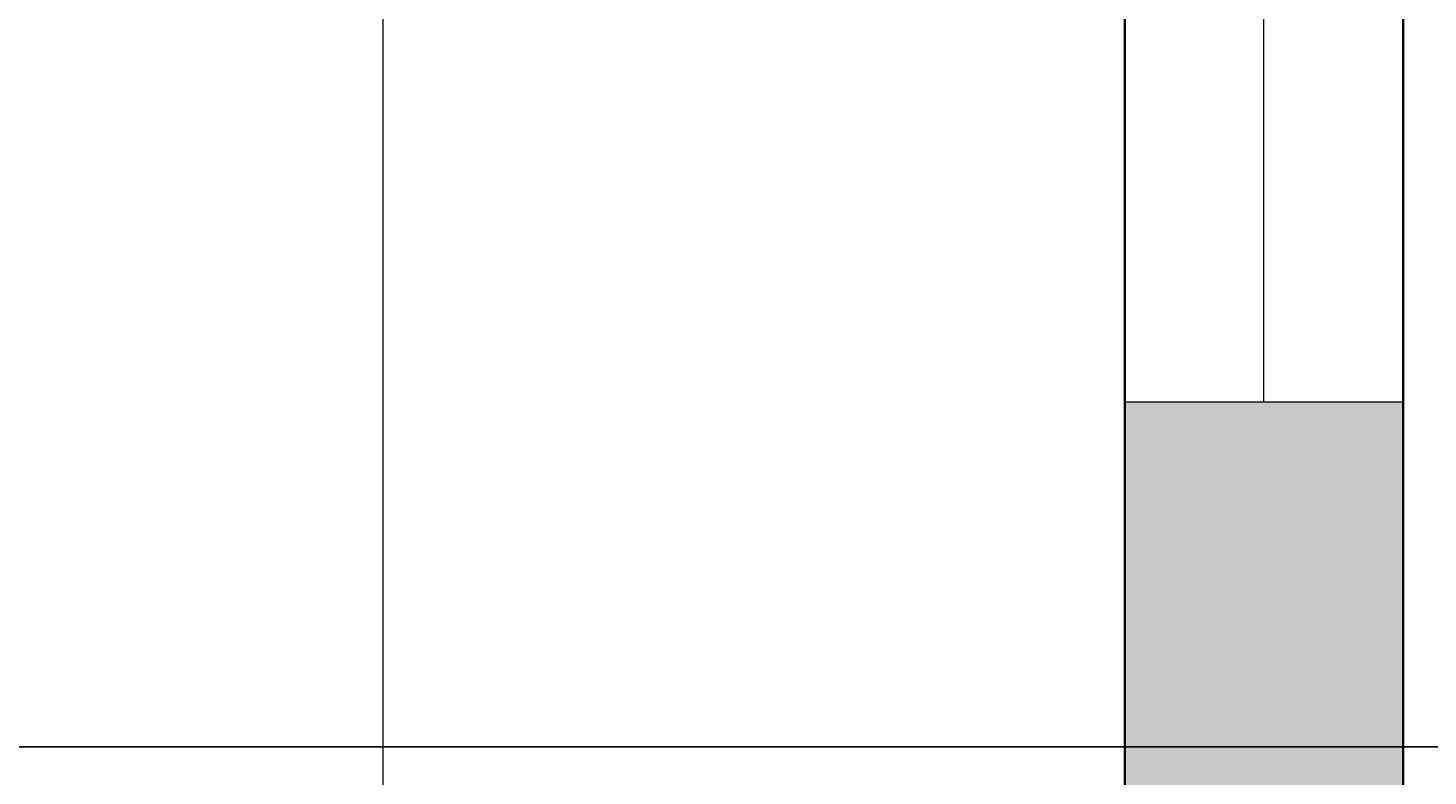
# Model space of a CAD drawing. Units: inches. Extents: x 1568 to 2529, y 2149 to 2897.
# Tile 9 of 16: x 1929 to 1974, y 2410 to 2434. Entities that reach past the tile are written whole.
import ezdxf

# ---------------------------------------------------------------- set-up
doc = ezdxf.new("R2010")
doc.units = ezdxf.units.IN
for name, color, linetype, lineweight in [('A-ANNO-DIMS', 2, 'Continuous', 18), ('A-FLOR-FIXT', 9, 'Continuous', 18), ('A-WALL-PATT', 172, 'Continuous', 13), ('wall', 7, 'Continuous', 35), ('window', 130, 'Continuous', 18)]:
    doc.layers.add(name, color=color, linetype=linetype, lineweight=lineweight)
doc.styles.get("Standard").update_dxf_attribs({"font": 'arial.ttf'})
doc.dimstyles.get("Standard").update_dxf_attribs({"dimtxt": 0.18, "dimasz": 0.18, "dimexe": 0.18, "dimexo": 0.0625, "dimgap": 0.09, "dimtad": 0, "dimtih": 1, "dimtoh": 1, "dimdec": 4, "dimzin": 0, "dimdsep": 46, "dimtxsty": 'Standard', "dimcen": 0.09, "dimadec": 0, "dimazin": 0, "dimtfac": 1, "dimtdec": 4, "dimtofl": 0, "dimtmove": 0, "dimatfit": 3, "dimfxl": 1, "dimtolj": 1, "dimtzin": 0, "dimarcsym": 0})

# ---------------------------------------------------------------- blocks, each defined once
blk = doc.blocks.new('*D28')
at = {"layer": 'A-ANNO-DIMS', "color": 0, "lineweight": -2, "transparency": 16777216}
for p, q in [((1973.643, 2801.532), (2009.61, 2801.532)), ((2009.43, 2801.352), (2009.43, 2501.714)), ((2009.43, 2201.712), (2009.43, 2501.35)), ((1973.613, 2201.532), (2009.61, 2201.532))]:
    blk.add_line(p, q, dxfattribs=at)
at = {"layer": 'A-ANNO-DIMS', "color": 0, "transparency": 16777216}
for points in [[(2009.4, 2801.352), (2009.46, 2801.352), (2009.43, 2801.532)], [(2009.4, 2201.712), (2009.46, 2201.712), (2009.43, 2201.532)]]:
    blk.add_solid(points, dxfattribs=at)
at = {"layer": 'Defpoints', "color": 0, "transparency": 16777216}
for p in [(1973.58, 2801.532), (2009.43, 2801.532), (1973.551, 2201.532)]:
    blk.add_point(p, dxfattribs=at)
at = {"layer": 'A-ANNO-DIMS', "color": 0, "transparency": 16777216, "insert": (2009.43, 2501.532), "char_height": 0.18, "attachment_point": 5}
blk.add_mtext('\\A1;600', dxfattribs=at)
blk = doc.blocks.new('*D32')
at = {"layer": 'A-ANNO-DIMS', "color": 0, "lineweight": -2, "transparency": 16777216}
for p, q in [((1964.551, 2792.469), (1964.551, 2165.502)), ((1904.551, 2753.401), (1904.551, 2165.502)), ((1904.731, 2165.682), (1934.332, 2165.682)), ((1964.371, 2165.682), (1934.77, 2165.682))]:
    blk.add_line(p, q, dxfattribs=at)
at = {"layer": 'A-ANNO-DIMS', "color": 0, "transparency": 16777216}
for points in [[(1904.731, 2165.712), (1904.731, 2165.652), (1904.551, 2165.682)], [(1964.371, 2165.712), (1964.371, 2165.652), (1964.551, 2165.682)]]:
    blk.add_solid(points, dxfattribs=at)
at = {"layer": 'Defpoints', "color": 0, "transparency": 16777216}
for p in [(1964.551, 2792.532), (1904.551, 2753.463), (1964.551, 2165.682)]:
    blk.add_point(p, dxfattribs=at)
at = {"layer": 'A-ANNO-DIMS', "color": 0, "transparency": 16777216, "insert": (1934.551, 2165.682), "char_height": 0.18, "attachment_point": 5}
blk.add_mtext('\\A1;60', dxfattribs=at)
blk = doc.blocks.new('*D35')
at = {"layer": 'A-ANNO-DIMS', "color": 0, "lineweight": -2, "transparency": 16777216}
for p, q in [((1759.113, 2451.227), (2009.61, 2451.227)), ((2009.43, 2451.047), (2009.43, 2431.409)), ((2009.43, 2411.407), (2009.43, 2431.045)), ((1759.113, 2411.227), (2009.61, 2411.227))]:
    blk.add_line(p, q, dxfattribs=at)
at = {"layer": 'A-ANNO-DIMS', "color": 0, "transparency": 16777216}
for points in [[(2009.4, 2451.047), (2009.46, 2451.047), (2009.43, 2451.227)], [(2009.4, 2411.407), (2009.46, 2411.407), (2009.43, 2411.227)]]:
    blk.add_solid(points, dxfattribs=at)
at = {"layer": 'Defpoints', "color": 0, "transparency": 16777216}
for p in [(1759.051, 2451.227), (2009.43, 2451.227), (1759.051, 2411.227)]:
    blk.add_point(p, dxfattribs=at)
at = {"layer": 'A-ANNO-DIMS', "color": 0, "transparency": 16777216, "insert": (2009.43, 2431.227), "char_height": 0.18, "attachment_point": 5}
blk.add_mtext('\\A1;40', dxfattribs=at)

msp = doc.modelspace()

# ---------------------------------------------------------------- hatches: boundary and pattern name
at = {"layer": 'A-WALL-PATT'}
h = msp.add_hatch(color=256, dxfattribs=at)
h.dxf.hatch_style = 1
h.paths.add_polyline_path([(1738.1593, 2801.532), (1634.4841, 2801.532), (1634.4841, 2792.532), (1738.1593, 2792.532)])
h.paths.add_polyline_path([(1812.4114, 2801.532), (1759.0925, 2801.532), (1759.0925, 2792.532), (1812.4114, 2792.532)])
h.paths.add_polyline_path([(1952.647, 2801.532), (1848.4114, 2801.532), (1848.4114, 2792.532), (1952.647, 2792.532)])
h.paths.add_polyline_path([(1973.5509, 2792.532), (1964.5509, 2792.532), (1964.5509, 2699.1671), (1973.5509, 2699.1671)])
h.paths.add_polyline_path([(1973.5509, 2663.1671), (1964.5509, 2663.1671), (1964.5509, 2630.5978), (1973.5509, 2630.5978)])
h.paths.add_polyline_path([(1973.5509, 2609.6646), (1964.5509, 2609.6646), (1964.5509, 2572.3679), (1973.5509, 2572.3679)])
h.paths.add_polyline_path([(1622.5509, 2753.3576), (1622.3864, 2753.3576), (1613.5509, 2753.3576), (1613.5509, 2705.9172), (1622.5509, 2705.9172)])
h.paths.add_polyline_path([(1622.5509, 2669.9172), (1613.5509, 2669.9172), (1613.5509, 2624.532), (1622.5509, 2624.532)])
h.paths.add_polyline_path([(1759.0509, 2757.9833), (1754.5509, 2757.9833), (1754.5509, 2744.532), (1622.5509, 2744.532), (1622.5509, 2740.032), (1754.5509, 2740.032), (1754.5509, 2730.8156), (1759.0509, 2730.8156), (1759.0509, 2740.032)])
h.paths.add_polyline_path([(1759.0509, 2690.8156), (1754.5509, 2690.8156), (1754.5509, 2624.532), (1759.0509, 2624.532)])
h.paths.add_polyline_path([(1738.1177, 2620.032), (1634.4841, 2620.032), (1634.4841, 2615.532), (1738.1177, 2615.532)])
h.paths.add_polyline_path([(1622.5509, 2615.532), (1613.5509, 2615.532), (1613.5509, 2564.2764), (1622.5509, 2564.2764)])
h.paths.add_polyline_path([(1759.0509, 2411.2271), (1754.5509, 2411.2271), (1754.5509, 2339.532), (1759.0509, 2339.532)])
h.paths.add_polyline_path([(1759.0509, 2464.032), (1734.3925, 2464.032), (1622.5509, 2464.032), (1622.5509, 2459.532), (1736.5509, 2459.532), (1754.5509, 2459.532), (1754.5509, 2451.2271), (1759.0509, 2451.2271)])
h.paths.add_polyline_path([(1844.5509, 2471.532), (1858.1805, 2471.532), (1858.1805, 2476.032), (1844.5509, 2476.032), (1844.5509, 2510.0763), (1840.0509, 2510.0763), (1840.0509, 2476.032), (1840.0509, 2339.532), (1844.5509, 2339.532)])
h.paths.add_polyline_path([(1844.5509, 2596.032), (1964.5509, 2596.032), (1964.5509, 2600.532), (1840.0509, 2600.532), (1840.0509, 2570.0763), (1844.5509, 2570.0763)])
h.paths.add_polyline_path([(1964.5509, 2476.032), (1894.1805, 2476.032), (1894.1805, 2471.532), (1964.5509, 2471.532)])
h.paths.add_polyline_path([(1622.5509, 2528.2764), (1613.5509, 2528.2764), (1613.5509, 2436.512), (1622.5509, 2436.512)])
h.paths.add_polyline_path([(1622.5509, 2400.512), (1613.5509, 2400.512), (1613.5509, 2339.532), (1622.5509, 2339.532)])
h.paths.add_polyline_path([(1738.9144, 2339.532), (1634.4841, 2339.532), (1634.4841, 2330.532), (1738.9144, 2330.532)])
h.paths.add_polyline_path([(1792.463, 2336.532, -0.0187698), (1792.5756, 2339.532), (1783.8928, 2339.532), (1783.8928, 2330.532), (1792.463, 2330.532)])
h.paths.add_polyline_path([(1952.6177, 2339.532), (1885.2912, 2339.532), (1885.2912, 2330.532), (1952.6177, 2330.532)])
h.paths.add_polyline_path([(1973.5509, 2422.371), (1964.5509, 2422.371), (1964.5509, 2395.032), (1964.5509, 2387.286), (1964.5509, 2339.532), (1973.5509, 2339.532)])
h.paths.add_polyline_path([(1973.5509, 2536.3679), (1964.5509, 2536.3679), (1964.5509, 2476.032), (1964.5509, 2458.371), (1973.5509, 2458.371)])

# ---------------------------------------------------------------- linework, layer by layer
at = {"layer": 'A-FLOR-FIXT'}
msp.add_line((1940.5509, 2471.532), (1940.5509, 2339.532), dxfattribs=at)
at = {"layer": 'wall'}
msp.add_line((1964.5509, 2387.286), (1964.5509, 2414.1822), dxfattribs=at)
msp.add_lwpolyline([(1613.5509, 2201.532), (1973.5509, 2201.532), (1973.5509, 2801.532), (1613.5509, 2801.532)], close=True, dxfattribs=at)
msp.add_lwpolyline([(1964.5509, 2395.032), (1964.5509, 2792.532), (1622.5509, 2792.532), (1622.5509, 2624.532)], dxfattribs=at)
at = {"layer": 'window'}
for p, q in [((1969.0509, 2422.371), (1969.0509, 2458.371)), ((1964.5509, 2422.371), (1973.5509, 2422.371))]:
    msp.add_line(p, q, dxfattribs=at)

# ---------------------------------------------------------------- dimensions: what is measured, and where the dimension line sits
at = {"layer": 'A-ANNO-DIMS'}
for base, p1, p2, picture, middle in [((2009.4302, 2801.532), (1973.5509, 2201.532), (1973.5802, 2801.532), '*D28', (2009.4302, 2501.532)), ((2009.4302, 2451.2271), (1759.0509, 2411.2271), (1759.0509, 2451.2271), '*D35', (2009.4302, 2431.2271))]:
    dim = msp.add_linear_dim(base=base, p1=p1, p2=p2, angle=90, dimstyle='Standard', override={"dimdec": 0, "dimlfac": 1, "dimrnd": 0, "dimzin": 0, "dimdsep": 46, "dimlunit": 2}, dxfattribs=at)
    dim.commit()
    dim.dimension.update_dxf_attribs({"geometry": picture, "text_midpoint": middle})
dim = msp.add_linear_dim(base=(1964.5509, 2165.682), p1=(1904.5509, 2753.4635), p2=(1964.5509, 2792.532), dimstyle='Standard', override={"dimdec": 0, "dimlfac": 1, "dimrnd": 0, "dimzin": 0, "dimdsep": 46, "dimlunit": 2}, dxfattribs=at)
dim.commit()
dim.dimension.update_dxf_attribs({"geometry": '*D32', "text_midpoint": (1934.5509, 2165.682)})

doc.saveas('drawing.dxf')
